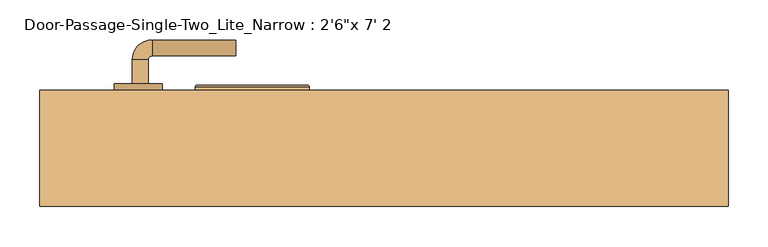
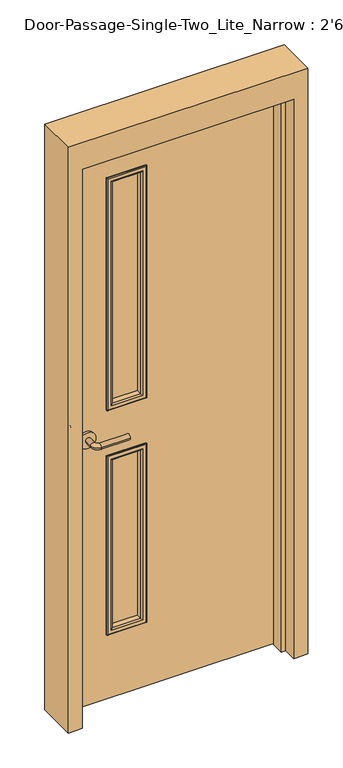
"""IFC4 building model written with IfcOpenShell, lengths in millimetres: door geometry."""

from ifc_helpers import new_model, si_unit, point, frame, frame_2d, origin, place, context, project, spatial, polyline, circle_curve, ellipse_curve, trimmed, segment, composite_curve, outline, extrude, faceted_brep, source, transform, mapped, element, save
from ifc_brep_helpers import plane_surface, cylinder_surface, revolved_surface, advanced_brep


def door_6f870c18(model_context):
    return source(origin(), model_context, "Body", "SolidModel", [
        advanced_brep(
        [(-315.990625, 42.8, 1016.0), (-295.990625, 42.8, 1016.0), (-295.990625, 12.8, 1016.0), (-315.990625, 12.8, 1016.0), (-290.990625, 7.8, 1016.0), (-290.990625, -12.2, 1016.0), (-185.990625, -12.2, 1016.0), (-185.990625, 7.8, 1016.0)],
        [
            (0, 1, circle_curve(frame((-305.990625, 42.8, 1016.0), z_axis=(0.0, 1.0, 0.0), x_axis=(1.0, 0.0, 0.0)), 10.0)),
            (1, 0, circle_curve(frame((-305.990625, 42.8, 1016.0), z_axis=(0.0, 1.0, 0.0), x_axis=(1.0, 0.0, 0.0)), 10.0)),
            (1, 2),
            (2, 3, circle_curve(frame((-305.990625, 12.8, 1016.0), z_axis=(0.0, 1.0, 0.0), x_axis=(1.0, 0.0, 0.0)), 10.0)),
            (3, 0),
            (3, 2, circle_curve(frame((-305.990625, 12.8, 1016.0), z_axis=(0.0, 1.0, 0.0), x_axis=(1.0, 0.0, 0.0)), 10.0)),
            (4, 5, circle_curve(frame((-290.990625, -2.2, 1016.0), z_axis=(-1.0, 0.0, 0.0), x_axis=(0.0, 1.0, 0.0)), 10.0)),
            (5, 3, circle_curve(frame((-290.990625, 12.8, 1016.0), z_axis=(0.0, 0.0, -1.0), x_axis=(-1.0, 0.0, 0.0)), 25.0)),
            (2, 4, circle_curve(frame((-290.990625, 12.8, 1016.0), z_axis=(0.0, 0.0, 1.0), x_axis=(-1.0, 0.0, 0.0)), 5.0)),
            (5, 4, circle_curve(frame((-290.990625, -2.2, 1016.0), z_axis=(-1.0, 0.0, 0.0), x_axis=(0.0, 1.0, 0.0)), 10.0)),
            (6, 7, circle_curve(frame((-185.990625, -2.2, 1016.0), z_axis=(1.0, 0.0, 0.0), x_axis=(0.0, 1.0, 0.0)), 10.0)),
            (7, 6, circle_curve(frame((-185.990625, -2.2, 1016.0), z_axis=(1.0, 0.0, 0.0), x_axis=(0.0, 1.0, 0.0)), 10.0)),
            (4, 7),
            (6, 5),
        ],
        [
            plane_surface(frame((-305.990625, 42.8, 1016.0), z_axis=(0.0, 1.0, 0.0), x_axis=(0.0, 0.0, 1.0))),
            cylinder_surface(frame((-305.990625, 42.8, 1016.0), z_axis=(0.0, 1.0, 0.0), x_axis=(1.0, 0.0, 0.0)), 10.0),
            revolved_surface(trimmed(ellipse_curve(frame((-305.990625, 12.8, 1016.0), z_axis=(0.0, -1.0, 0.0), x_axis=(1.0, 0.0, 0.0)), 10.0, 10.0), [point((-315.990625, 12.8, 1016.0))], [point((-295.990625, 12.8, 1016.0))], True, "CARTESIAN"), (-290.990625, 12.8, 1016.0), (0.0, 0.0, -1.0)),
            revolved_surface(trimmed(ellipse_curve(frame((-305.990625, 12.8, 1016.0), z_axis=(0.0, -1.0, 0.0), x_axis=(1.0, 0.0, 0.0)), 10.0, 10.0), [point((-295.990625, 12.8, 1016.0))], [point((-315.990625, 12.8, 1016.0))], True, "CARTESIAN"), (-290.990625, 12.8, 1016.0), (0.0, 0.0, -1.0)),
            plane_surface(frame((-185.990625, -2.2, 1016.0), z_axis=(1.0, 0.0, 0.0), x_axis=(0.0, 0.0, 1.0))),
            cylinder_surface(frame((-290.990625, -2.2, 1016.0), z_axis=(-1.0, 0.0, 0.0), x_axis=(0.0, 1.0, 0.0)), 10.0),
        ],
        [
            (0, [[1, 2]]),
            (1, [[3, 4, 5, -2]]),
            (1, [[-5, 6, -3, -1]]),
            (2, [[7, 8, -4, 9]]),
            (3, [[10, -9, -6, -8]]),
            (4, [[11, 12]]),
            (5, [[13, -11, 14, -7]]),
            (5, [[-14, -12, -13, -10]]),
        ],
    ),
        extrude(outline(composite_curve([segment(trimmed(circle_curve(frame_2d((1016.0, -308.490625)), 30.0), [point((1016.0, -338.490625))], [point((1016.0, -278.490625))], False, "CARTESIAN"), True, "CONTINUOUS"), segment(trimmed(circle_curve(frame_2d((1016.0, -308.490625)), 30.0), [point((1016.0, -278.490625))], [point((1016.0, -338.490625))], False, "CARTESIAN"), True, "CONTINUOUS")], self_intersect=False)), frame((0.0, 42.8, 0.0), z_axis=(0.0, 1.0, 0.0), x_axis=(0.0, 0.0, 1.0)), (0.0, 0.0, 1.0), 8.0),
        advanced_brep(
        [(-315.990625, 103.25, 1016.0), (-295.990625, 103.25, 1016.0), (-315.990625, 133.25, 1016.0), (-295.990625, 133.25, 1016.0), (-290.990625, 138.25, 1016.0), (-290.990625, 158.25, 1016.0), (-185.990625, 158.25, 1016.0), (-185.990625, 138.25, 1016.0)],
        [
            (0, 1, circle_curve(frame((-305.990625, 103.25, 1016.0), z_axis=(0.0, -1.0, 0.0), x_axis=(1.0, 0.0, 0.0)), 10.0)),
            (1, 0, circle_curve(frame((-305.990625, 103.25, 1016.0), z_axis=(0.0, -1.0, 0.0), x_axis=(1.0, 0.0, 0.0)), 10.0)),
            (0, 2),
            (2, 3, circle_curve(frame((-305.990625, 133.25, 1016.0), z_axis=(0.0, -1.0, 0.0), x_axis=(1.0, 0.0, 0.0)), 10.0)),
            (3, 1),
            (3, 2, circle_curve(frame((-305.990625, 133.25, 1016.0), z_axis=(0.0, -1.0, 0.0), x_axis=(1.0, 0.0, 0.0)), 10.0)),
            (4, 3, circle_curve(frame((-290.990625, 133.25, 1016.0), z_axis=(0.0, 0.0, 1.0), x_axis=(-1.0, 0.0, 0.0)), 5.0)),
            (2, 5, circle_curve(frame((-290.990625, 133.25, 1016.0), z_axis=(0.0, 0.0, -1.0), x_axis=(-1.0, 0.0, 0.0)), 25.0)),
            (5, 4, circle_curve(frame((-290.990625, 148.25, 1016.0), z_axis=(-1.0, 0.0, 0.0), x_axis=(0.0, -1.0, 0.0)), 10.0)),
            (4, 5, circle_curve(frame((-290.990625, 148.25, 1016.0), z_axis=(-1.0, 0.0, 0.0), x_axis=(0.0, -1.0, 0.0)), 10.0)),
            (6, 7, circle_curve(frame((-185.990625, 148.25, 1016.0), z_axis=(1.0, 0.0, 0.0), x_axis=(0.0, -1.0, 0.0)), 10.0)),
            (7, 6, circle_curve(frame((-185.990625, 148.25, 1016.0), z_axis=(1.0, 0.0, 0.0), x_axis=(0.0, -1.0, 0.0)), 10.0)),
            (5, 6),
            (7, 4),
        ],
        [
            plane_surface(frame((-305.990625, 103.25, 1016.0), z_axis=(0.0, -1.0, 0.0), x_axis=(0.0, 0.0, 1.0))),
            cylinder_surface(frame((-305.990625, 103.25, 1016.0), z_axis=(0.0, -1.0, 0.0), x_axis=(1.0, 0.0, 0.0)), 10.0),
            revolved_surface(trimmed(ellipse_curve(frame((-305.990625, 133.25, 1016.0), z_axis=(0.0, -1.0, 0.0), x_axis=(1.0, 0.0, 0.0)), 10.0, 10.0), [point((-315.990625, 133.25, 1016.0))], [point((-295.990625, 133.25, 1016.0))], True, "CARTESIAN"), (-290.990625, 133.25, 1016.0), (0.0, 0.0, -1.0)),
            revolved_surface(trimmed(ellipse_curve(frame((-305.990625, 133.25, 1016.0), z_axis=(0.0, -1.0, 0.0), x_axis=(1.0, 0.0, 0.0)), 10.0, 10.0), [point((-295.990625, 133.25, 1016.0))], [point((-315.990625, 133.25, 1016.0))], True, "CARTESIAN"), (-290.990625, 133.25, 1016.0), (0.0, 0.0, -1.0)),
            plane_surface(frame((-185.990625, 148.25, 1016.0), z_axis=(1.0, 0.0, 0.0), x_axis=(0.0, 0.0, 1.0))),
            cylinder_surface(frame((-290.990625, 148.25, 1016.0), z_axis=(-1.0, 0.0, 0.0), x_axis=(0.0, -1.0, 0.0)), 10.0),
        ],
        [
            (0, [[1, 2]]),
            (1, [[-1, 3, 4, 5]]),
            (1, [[-2, -5, 6, -3]]),
            (2, [[7, -4, 8, 9]]),
            (3, [[-8, -6, -7, 10]]),
            (4, [[11, 12]]),
            (5, [[-9, 13, -12, 14]]),
            (5, [[-10, -14, -11, -13]]),
        ],
    ),
        extrude(outline(composite_curve([segment(trimmed(circle_curve(frame_2d((1016.0, -308.490625)), 30.0), [point((1016.0, -338.490625))], [point((1016.0, -278.490625))], False, "CARTESIAN"), True, "CONTINUOUS"), segment(trimmed(circle_curve(frame_2d((1016.0, -308.490625)), 30.0), [point((1016.0, -278.490625))], [point((1016.0, -338.490625))], False, "CARTESIAN"), True, "CONTINUOUS")], self_intersect=False)), frame((0.0, 95.25, 0.0), z_axis=(0.0, 1.0, 0.0), x_axis=(0.0, 0.0, 1.0)), (0.0, 0.0, 1.0), 8.0),
        extrude(outline(polyline([(2133.6, -381.0), (0.0, -381.0), (0.0, 381.0), (2133.6, 381.0), (2133.6, -381.0)]), holes=[polyline([(1981.2, -228.6), (1981.2, -101.6), (1111.25, -101.6), (1111.25, -228.6), (1981.2, -228.6)]), polyline([(920.75, -228.6), (920.75, -101.6), (254.0, -101.6), (254.0, -228.6), (920.75, -228.6)])]), frame((0.0, 50.8, 0.0), z_axis=(0.0, 1.0, 0.0), x_axis=(0.0, 0.0, 1.0)), (0.0, 0.0, 1.0), 44.45),
        faceted_brep([(381.0, 46.0375, 0.0), (381.0, 95.25, 0.0), (431.8, 95.25, 0.0), (431.8, -50.8, 0.0), (381.0, -50.8, 0.0), (381.0, -1.5875, 0.0), (365.125, -1.5875, 0.0), (365.125, 46.0375, 0.0), (381.0, 46.0375, 2133.6), (381.0, 95.25, 2133.6), (-381.0, 95.25, 2133.6), (-381.0, 95.25, 0.0), (-431.8, 95.25, 0.0), (-431.8, 95.25, 2235.2), (431.8, 95.25, 2235.2), (431.8, -50.8, 2235.2), (-431.8, -50.8, 2235.2), (-431.8, -50.8, 0.0), (-381.0, -50.8, 0.0), (-381.0, -50.8, 2133.6), (381.0, -50.8, 2133.6), (381.0, -1.5875, 2133.6), (-381.0, -1.5875, 2133.6), (-381.0, -1.5875, 0.0), (-365.125, -1.5875, 0.0), (-365.125, -1.5875, 2117.725), (365.125, -1.5875, 2117.725), (365.125, 46.0375, 2117.725), (-365.125, 46.0375, 2117.725), (-365.125, 46.0375, 0.0), (-381.0, 46.0375, 0.0), (-381.0, 46.0375, 2133.6)], [[[0, 1, 2, 3, 4, 5, 6, 7]], [[1, 0, 8, 9]], [[2, 1, 9, 10, 11, 12, 13, 14]], [[3, 2, 14, 15]], [[4, 3, 15, 16, 17, 18, 19, 20]], [[5, 4, 20, 21]], [[6, 5, 21, 22, 23, 24, 25, 26]], [[7, 6, 26, 27]], [[0, 7, 27, 28, 29, 30, 31, 8]], [[9, 8, 31, 10]], [[20, 19, 22, 21]], [[26, 25, 28, 27]], [[12, 11, 30, 29, 24, 23, 18, 17]], [[11, 10, 31, 30]], [[13, 12, 17, 16]], [[19, 18, 23, 22]], [[25, 24, 29, 28]], [[15, 14, 13, 16]]]),
        extrude(outline(polyline([(-101.6, 69.85), (-228.6, 69.85), (-228.6, 76.2), (-101.6, 76.2), (-101.6, 69.85)])), frame((0.0, 0.0, 1111.25), z_axis=(0.0, 0.0, 1.0), x_axis=(1.0, 0.0, 0.0)), (0.0, 0.0, 1.0), 869.95),
        extrude(outline(polyline([(-101.6, 69.85), (-228.6, 69.85), (-228.6, 76.2), (-101.6, 76.2), (-101.6, 69.85)])), frame((0.0, 0.0, 254.0), z_axis=(0.0, 0.0, 1.0), x_axis=(1.0, 0.0, 0.0)), (0.0, 0.0, 1.0), 666.75),
        advanced_brep(
        [(-228.6, 76.2, 1981.2), (-228.6, 95.25, 1981.2), (-228.6, 95.25, 1111.25), (-228.6, 76.2, 1111.25), (-216.6, 96.25, 1969.2), (-216.6, 76.2, 1969.2), (-216.6, 76.2, 1123.25), (-216.6, 96.25, 1123.25), (-221.6, 101.25, 1974.2), (-221.6, 101.25, 1118.25), (-236.6, 99.25, 1989.2), (-234.6, 101.25, 1987.2), (-234.6, 101.25, 1105.25), (-236.6, 99.25, 1103.25), (-236.6, 95.25, 1989.2), (-236.6, 95.25, 1103.25), (-101.6, 95.25, 1111.25), (-101.6, 76.2, 1111.25), (-113.6, 76.2, 1123.25), (-113.6, 96.25, 1123.25), (-108.6, 101.25, 1118.25), (-95.6, 101.25, 1105.25), (-93.6, 99.25, 1103.25), (-93.6, 95.25, 1103.25), (-101.6, 95.25, 1981.2), (-101.6, 76.2, 1981.2), (-113.6, 76.2, 1969.2), (-113.6, 96.25, 1969.2), (-108.6, 101.25, 1974.2), (-95.6, 101.25, 1987.2), (-93.6, 99.25, 1989.2), (-93.6, 95.25, 1989.2)],
        [
            (0, 1),
            (1, 2),
            (2, 3),
            (3, 0),
            (4, 5),
            (5, 6),
            (6, 7),
            (7, 4),
            (8, 4, ellipse_curve(frame((-221.6, 96.25, 1974.2), z_axis=(-0.7071067811865475, 0.0, -0.7071067811865475), x_axis=(-0.7071067811865474, 0.0, 0.7071067811865476)), 7.0710678, 5.0)),
            (7, 9, ellipse_curve(frame((-221.6, 96.25, 1118.25), z_axis=(-0.7071067811865475, 0.0, 0.7071067811865475), x_axis=(0.7071067811865474, 0.0, 0.7071067811865476)), 7.0710678, 5.0)),
            (9, 8),
            (10, 11, ellipse_curve(frame((-234.6, 99.25, 1987.2), z_axis=(-0.7071067811865475, 0.0, -0.7071067811865475), x_axis=(-0.7071067811865474, 0.0, 0.7071067811865476)), 2.8284271, 2.0)),
            (11, 12),
            (12, 13, ellipse_curve(frame((-234.6, 99.25, 1105.25), z_axis=(-0.7071067811865475, 0.0, 0.7071067811865475), x_axis=(0.7071067811865474, 0.0, 0.7071067811865476)), 2.8284271, 2.0)),
            (13, 10),
            (14, 10),
            (13, 15),
            (15, 14),
            (2, 16),
            (16, 17),
            (17, 3),
            (6, 18),
            (18, 19),
            (19, 7),
            (19, 20, ellipse_curve(frame((-108.6, 96.25, 1118.25), z_axis=(-0.7071067811865475, 0.0, -0.7071067811865475), x_axis=(-0.7071067811865476, 0.0, 0.7071067811865474)), 7.0710678, 5.0)),
            (20, 9),
            (12, 21),
            (21, 22, ellipse_curve(frame((-95.6, 99.25, 1105.25), z_axis=(-0.7071067811865475, 0.0, -0.7071067811865475), x_axis=(-0.7071067811865476, 0.0, 0.7071067811865474)), 2.8284271, 2.0)),
            (22, 13),
            (22, 23),
            (23, 15),
            (16, 24),
            (24, 25),
            (25, 17),
            (18, 26),
            (26, 27),
            (27, 19),
            (27, 28, ellipse_curve(frame((-108.6, 96.25, 1974.2), z_axis=(0.7071067811865475, 0.0, -0.7071067811865475), x_axis=(-0.7071067811865474, 0.0, -0.7071067811865476)), 7.0710678, 5.0)),
            (28, 20),
            (21, 29),
            (29, 30, ellipse_curve(frame((-95.6, 99.25, 1987.2), z_axis=(0.7071067811865475, 0.0, -0.7071067811865475), x_axis=(-0.7071067811865474, 0.0, -0.7071067811865476)), 2.8284271, 2.0)),
            (30, 22),
            (30, 31),
            (31, 23),
            (31, 14),
            (1, 24),
            (0, 25),
            (5, 26),
            (4, 27),
            (8, 28),
            (11, 29),
            (10, 30),
        ],
        [
            plane_surface(frame((-228.6, 95.25, 1981.2), z_axis=(-1.0, 0.0, 0.0), x_axis=(0.0, 0.0, -1.0))),
            plane_surface(frame((-216.6, 76.2, 1969.2), z_axis=(1.0, 0.0, 0.0), x_axis=(0.0, 0.0, -1.0))),
            cylinder_surface(frame((-221.6, 96.25, 1981.2), z_axis=(0.0, 0.0, 1.0), x_axis=(-1.0, 0.0, 0.0)), 5.0),
            cylinder_surface(frame((-234.6, 99.25, 1981.2), z_axis=(0.0, 0.0, 1.0), x_axis=(-1.0, 0.0, 0.0)), 2.0),
            plane_surface(frame((-236.6, 99.25, 1989.2), z_axis=(-1.0, 0.0, 0.0), x_axis=(0.0, 0.0, -1.0))),
            plane_surface(frame((-228.6, 95.25, 1111.25), z_axis=(0.0, 0.0, -1.0), x_axis=(1.0, 0.0, 0.0))),
            plane_surface(frame((-216.6, 76.2, 1123.25), z_axis=(0.0, 0.0, 1.0), x_axis=(1.0, 0.0, 0.0))),
            cylinder_surface(frame((-228.6, 96.25, 1118.25), z_axis=(-1.0, 0.0, 0.0), x_axis=(0.0, 0.0, -1.0)), 5.0),
            cylinder_surface(frame((-228.6, 99.25, 1105.25), z_axis=(-1.0, 0.0, 0.0), x_axis=(0.0, 0.0, -1.0)), 2.0),
            plane_surface(frame((-236.6, 99.25, 1103.25), z_axis=(0.0, 0.0, -1.0), x_axis=(1.0, 0.0, 0.0))),
            plane_surface(frame((-101.6, 95.25, 1111.25), z_axis=(1.0, 0.0, 0.0), x_axis=(0.0, 0.0, 1.0))),
            plane_surface(frame((-113.6, 76.2, 1123.25), z_axis=(-1.0, 0.0, 0.0), x_axis=(0.0, 0.0, 1.0))),
            cylinder_surface(frame((-108.6, 96.25, 1111.25), z_axis=(0.0, 0.0, -1.0), x_axis=(1.0, 0.0, 0.0)), 5.0),
            cylinder_surface(frame((-95.6, 99.25, 1111.25), z_axis=(0.0, 0.0, -1.0), x_axis=(1.0, 0.0, 0.0)), 2.0),
            plane_surface(frame((-93.6, 99.25, 1103.25), z_axis=(1.0, 0.0, 0.0), x_axis=(0.0, 0.0, 1.0))),
            plane_surface(frame((-93.6, 95.25, 1989.2), z_axis=(0.0, -1.0, 0.0), x_axis=(-1.0, 0.0, 0.0))),
            plane_surface(frame((-101.6, 95.25, 1981.2), z_axis=(0.0, 0.0, 1.0), x_axis=(-1.0, 0.0, 0.0))),
            plane_surface(frame((-101.6, 76.2, 1981.2), z_axis=(0.0, -1.0, 0.0), x_axis=(-1.0, 0.0, 0.0))),
            plane_surface(frame((-113.6, 76.2, 1969.2), z_axis=(0.0, 0.0, -1.0), x_axis=(-1.0, 0.0, 0.0))),
            cylinder_surface(frame((-101.6, 96.25, 1974.2), z_axis=(1.0, 0.0, 0.0), x_axis=(0.0, 0.0, 1.0)), 5.0),
            plane_surface(frame((-108.6, 101.25, 1974.2), z_axis=(0.0, 1.0, 0.0), x_axis=(-1.0, 0.0, 0.0))),
            cylinder_surface(frame((-101.6, 99.25, 1987.2), z_axis=(1.0, 0.0, 0.0), x_axis=(0.0, 0.0, 1.0)), 2.0),
            plane_surface(frame((-93.6, 99.25, 1989.2), z_axis=(0.0, 0.0, 1.0), x_axis=(-1.0, 0.0, 0.0))),
        ],
        [
            (0, [[1, 2, 3, 4]]),
            (1, [[5, 6, 7, 8]]),
            (2, [[9, -8, 10, 11]]),
            (3, [[12, 13, 14, 15]]),
            (4, [[16, -15, 17, 18]]),
            (5, [[-3, 19, 20, 21]]),
            (6, [[-7, 22, 23, 24]]),
            (7, [[-10, -24, 25, 26]]),
            (8, [[-14, 27, 28, 29]]),
            (9, [[-17, -29, 30, 31]]),
            (10, [[-20, 32, 33, 34]]),
            (11, [[-23, 35, 36, 37]]),
            (12, [[-25, -37, 38, 39]]),
            (13, [[-28, 40, 41, 42]]),
            (14, [[-30, -42, 43, 44]]),
            (15, [[-31, -44, 45, -18], [46, -32, -19, -2]]),
            (16, [[-33, -46, -1, 47]]),
            (17, [[-21, -34, -47, -4], [48, -35, -22, -6]]),
            (18, [[-36, -48, -5, 49]]),
            (19, [[-38, -49, -9, 50]]),
            (20, [[51, -40, -27, -13], [-26, -39, -50, -11]]),
            (21, [[-41, -51, -12, 52]]),
            (22, [[-43, -52, -16, -45]]),
        ],
    ),
        advanced_brep(
        [(-228.6, 69.85, 1111.25), (-228.6, 50.8, 1111.25), (-228.6, 50.8, 1981.2), (-228.6, 69.85, 1981.2), (-216.6, 49.8, 1123.25), (-216.6, 69.85, 1123.25), (-216.6, 69.85, 1969.2), (-216.6, 49.8, 1969.2), (-221.6, 44.8, 1118.25), (-221.6, 44.8, 1974.2), (-236.6, 46.8, 1103.25), (-234.6, 44.8, 1105.25), (-234.6, 44.8, 1987.2), (-236.6, 46.8, 1989.2), (-236.6, 50.8, 1103.25), (-236.6, 50.8, 1989.2), (-101.6, 50.8, 1981.2), (-101.6, 69.85, 1981.2), (-113.6, 69.85, 1969.2), (-113.6, 49.8, 1969.2), (-108.6, 44.8, 1974.2), (-95.6, 44.8, 1987.2), (-93.6, 46.8, 1989.2), (-93.6, 50.8, 1989.2), (-101.6, 50.8, 1111.25), (-101.6, 69.85, 1111.25), (-113.6, 69.85, 1123.25), (-113.6, 49.8, 1123.25), (-108.6, 44.8, 1118.25), (-95.6, 44.8, 1105.25), (-93.6, 46.8, 1103.25), (-93.6, 50.8, 1103.25)],
        [
            (0, 1),
            (1, 2),
            (2, 3),
            (3, 0),
            (4, 5),
            (5, 6),
            (6, 7),
            (7, 4),
            (8, 4, ellipse_curve(frame((-221.6, 49.8, 1118.25), z_axis=(-0.7071067811865475, 0.0, 0.7071067811865475), x_axis=(-0.7071067811865474, 0.0, -0.7071067811865476)), 7.0710678, 5.0)),
            (7, 9, ellipse_curve(frame((-221.6, 49.8, 1974.2), z_axis=(-0.7071067811865475, 0.0, -0.7071067811865475), x_axis=(0.7071067811865474, 0.0, -0.7071067811865476)), 7.0710678, 5.0)),
            (9, 8),
            (10, 11, ellipse_curve(frame((-234.6, 46.8, 1105.25), z_axis=(-0.7071067811865475, 0.0, 0.7071067811865475), x_axis=(-0.7071067811865474, 0.0, -0.7071067811865476)), 2.8284271, 2.0)),
            (11, 12),
            (12, 13, ellipse_curve(frame((-234.6, 46.8, 1987.2), z_axis=(-0.7071067811865475, 0.0, -0.7071067811865475), x_axis=(0.7071067811865474, 0.0, -0.7071067811865476)), 2.8284271, 2.0)),
            (13, 10),
            (14, 10),
            (13, 15),
            (15, 14),
            (2, 16),
            (16, 17),
            (17, 3),
            (6, 18),
            (18, 19),
            (19, 7),
            (19, 20, ellipse_curve(frame((-108.6, 49.8, 1974.2), z_axis=(-0.7071067811865475, 0.0, 0.7071067811865475), x_axis=(-0.7071067811865476, 0.0, -0.7071067811865474)), 7.0710678, 5.0)),
            (20, 9),
            (12, 21),
            (21, 22, ellipse_curve(frame((-95.6, 46.8, 1987.2), z_axis=(-0.7071067811865475, 0.0, 0.7071067811865475), x_axis=(-0.7071067811865476, 0.0, -0.7071067811865474)), 2.8284271, 2.0)),
            (22, 13),
            (22, 23),
            (23, 15),
            (16, 24),
            (24, 25),
            (25, 17),
            (18, 26),
            (26, 27),
            (27, 19),
            (27, 28, ellipse_curve(frame((-108.6, 49.8, 1118.25), z_axis=(0.7071067811865475, 0.0, 0.7071067811865475), x_axis=(-0.7071067811865474, 0.0, 0.7071067811865476)), 7.0710678, 5.0)),
            (28, 20),
            (21, 29),
            (29, 30, ellipse_curve(frame((-95.6, 46.8, 1105.25), z_axis=(0.7071067811865475, 0.0, 0.7071067811865475), x_axis=(-0.7071067811865474, 0.0, 0.7071067811865476)), 2.8284271, 2.0)),
            (30, 22),
            (30, 31),
            (31, 23),
            (31, 14),
            (1, 24),
            (0, 25),
            (5, 26),
            (4, 27),
            (8, 28),
            (11, 29),
            (10, 30),
        ],
        [
            plane_surface(frame((-228.6, 50.8, 1111.25), z_axis=(-1.0, 0.0, 0.0), x_axis=(0.0, 0.0, 1.0))),
            plane_surface(frame((-216.6, 69.85, 1123.25), z_axis=(1.0, 0.0, 0.0), x_axis=(0.0, 0.0, 1.0))),
            cylinder_surface(frame((-221.6, 49.8, 1111.25), z_axis=(0.0, 0.0, -1.0), x_axis=(-1.0, 0.0, 0.0)), 5.0),
            cylinder_surface(frame((-234.6, 46.8, 1111.25), z_axis=(0.0, 0.0, -1.0), x_axis=(-1.0, 0.0, 0.0)), 2.0),
            plane_surface(frame((-236.6, 46.8, 1103.25), z_axis=(-1.0, 0.0, 0.0), x_axis=(0.0, 0.0, 1.0))),
            plane_surface(frame((-228.6, 50.8, 1981.2), z_axis=(0.0, 0.0, 1.0), x_axis=(1.0, 0.0, 0.0))),
            plane_surface(frame((-216.6, 69.85, 1969.2), z_axis=(0.0, 0.0, -1.0), x_axis=(1.0, 0.0, 0.0))),
            cylinder_surface(frame((-228.6, 49.8, 1974.2), z_axis=(-1.0, 0.0, 0.0), x_axis=(0.0, 0.0, 1.0)), 5.0),
            cylinder_surface(frame((-228.6, 46.8, 1987.2), z_axis=(-1.0, 0.0, 0.0), x_axis=(0.0, 0.0, 1.0)), 2.0),
            plane_surface(frame((-236.6, 46.8, 1989.2), z_axis=(0.0, 0.0, 1.0), x_axis=(1.0, 0.0, 0.0))),
            plane_surface(frame((-101.6, 50.8, 1981.2), z_axis=(1.0, 0.0, 0.0), x_axis=(0.0, 0.0, -1.0))),
            plane_surface(frame((-113.6, 69.85, 1969.2), z_axis=(-1.0, 0.0, 0.0), x_axis=(0.0, 0.0, -1.0))),
            cylinder_surface(frame((-108.6, 49.8, 1981.2), z_axis=(0.0, 0.0, 1.0), x_axis=(1.0, 0.0, 0.0)), 5.0),
            cylinder_surface(frame((-95.6, 46.8, 1981.2), z_axis=(0.0, 0.0, 1.0), x_axis=(1.0, 0.0, 0.0)), 2.0),
            plane_surface(frame((-93.6, 46.8, 1989.2), z_axis=(1.0, 0.0, 0.0), x_axis=(0.0, 0.0, -1.0))),
            plane_surface(frame((-93.6, 50.8, 1103.25), z_axis=(0.0, 1.0, 0.0), x_axis=(-1.0, 0.0, 0.0))),
            plane_surface(frame((-101.6, 50.8, 1111.25), z_axis=(0.0, 0.0, -1.0), x_axis=(-1.0, 0.0, 0.0))),
            plane_surface(frame((-101.6, 69.85, 1111.25), z_axis=(0.0, 1.0, 0.0), x_axis=(-1.0, 0.0, 0.0))),
            plane_surface(frame((-113.6, 69.85, 1123.25), z_axis=(0.0, 0.0, 1.0), x_axis=(-1.0, 0.0, 0.0))),
            cylinder_surface(frame((-101.6, 49.8, 1118.25), z_axis=(1.0, 0.0, 0.0), x_axis=(0.0, 0.0, -1.0)), 5.0),
            plane_surface(frame((-108.6, 44.8, 1118.25), z_axis=(0.0, -1.0, 0.0), x_axis=(-1.0, 0.0, 0.0))),
            cylinder_surface(frame((-101.6, 46.8, 1105.25), z_axis=(1.0, 0.0, 0.0), x_axis=(0.0, 0.0, -1.0)), 2.0),
            plane_surface(frame((-93.6, 46.8, 1103.25), z_axis=(0.0, 0.0, -1.0), x_axis=(-1.0, 0.0, 0.0))),
        ],
        [
            (0, [[1, 2, 3, 4]]),
            (1, [[5, 6, 7, 8]]),
            (2, [[9, -8, 10, 11]]),
            (3, [[12, 13, 14, 15]]),
            (4, [[16, -15, 17, 18]]),
            (5, [[-3, 19, 20, 21]]),
            (6, [[-7, 22, 23, 24]]),
            (7, [[-10, -24, 25, 26]]),
            (8, [[-14, 27, 28, 29]]),
            (9, [[-17, -29, 30, 31]]),
            (10, [[-20, 32, 33, 34]]),
            (11, [[-23, 35, 36, 37]]),
            (12, [[-25, -37, 38, 39]]),
            (13, [[-28, 40, 41, 42]]),
            (14, [[-30, -42, 43, 44]]),
            (15, [[-31, -44, 45, -18], [46, -32, -19, -2]]),
            (16, [[-33, -46, -1, 47]]),
            (17, [[-21, -34, -47, -4], [48, -35, -22, -6]]),
            (18, [[-36, -48, -5, 49]]),
            (19, [[-38, -49, -9, 50]]),
            (20, [[51, -40, -27, -13], [-26, -39, -50, -11]]),
            (21, [[-41, -51, -12, 52]]),
            (22, [[-43, -52, -16, -45]]),
        ],
    ),
        advanced_brep(
        [(-228.6, 76.2, 920.75), (-228.6, 95.25, 920.75), (-228.6, 95.25, 254.0), (-228.6, 76.2, 254.0), (-216.6, 96.25, 908.75), (-216.6, 76.2, 908.75), (-216.6, 76.2, 266.0), (-216.6, 96.25, 266.0), (-221.6, 101.25, 913.75), (-221.6, 101.25, 261.0), (-236.6, 99.25, 928.75), (-234.6, 101.25, 926.75), (-234.6, 101.25, 248.0), (-236.6, 99.25, 246.0), (-236.6, 95.25, 928.75), (-236.6, 95.25, 246.0), (-101.6, 95.25, 254.0), (-101.6, 76.2, 254.0), (-113.6, 76.2, 266.0), (-113.6, 96.25, 266.0), (-108.6, 101.25, 261.0), (-95.6, 101.25, 248.0), (-93.6, 99.25, 246.0), (-93.6, 95.25, 246.0), (-101.6, 95.25, 920.75), (-101.6, 76.2, 920.75), (-113.6, 76.2, 908.75), (-113.6, 96.25, 908.75), (-108.6, 101.25, 913.75), (-95.6, 101.25, 926.75), (-93.6, 99.25, 928.75), (-93.6, 95.25, 928.75)],
        [
            (0, 1),
            (1, 2),
            (2, 3),
            (3, 0),
            (4, 5),
            (5, 6),
            (6, 7),
            (7, 4),
            (8, 4, ellipse_curve(frame((-221.6, 96.25, 913.75), z_axis=(-0.7071067811865475, 0.0, -0.7071067811865475), x_axis=(-0.7071067811865474, 0.0, 0.7071067811865476)), 7.0710678, 5.0)),
            (7, 9, ellipse_curve(frame((-221.6, 96.25, 261.0), z_axis=(-0.7071067811865475, 0.0, 0.7071067811865475), x_axis=(0.7071067811865474, 0.0, 0.7071067811865476)), 7.0710678, 5.0)),
            (9, 8),
            (10, 11, ellipse_curve(frame((-234.6, 99.25, 926.75), z_axis=(-0.7071067811865475, 0.0, -0.7071067811865475), x_axis=(-0.7071067811865474, 0.0, 0.7071067811865476)), 2.8284271, 2.0)),
            (11, 12),
            (12, 13, ellipse_curve(frame((-234.6, 99.25, 248.0), z_axis=(-0.7071067811865475, 0.0, 0.7071067811865475), x_axis=(0.7071067811865474, 0.0, 0.7071067811865476)), 2.8284271, 2.0)),
            (13, 10),
            (14, 10),
            (13, 15),
            (15, 14),
            (2, 16),
            (16, 17),
            (17, 3),
            (6, 18),
            (18, 19),
            (19, 7),
            (19, 20, ellipse_curve(frame((-108.6, 96.25, 261.0), z_axis=(-0.7071067811865475, 0.0, -0.7071067811865475), x_axis=(-0.7071067811865476, 0.0, 0.7071067811865474)), 7.0710678, 5.0)),
            (20, 9),
            (12, 21),
            (21, 22, ellipse_curve(frame((-95.6, 99.25, 248.0), z_axis=(-0.7071067811865475, 0.0, -0.7071067811865475), x_axis=(-0.7071067811865476, 0.0, 0.7071067811865474)), 2.8284271, 2.0)),
            (22, 13),
            (22, 23),
            (23, 15),
            (16, 24),
            (24, 25),
            (25, 17),
            (18, 26),
            (26, 27),
            (27, 19),
            (27, 28, ellipse_curve(frame((-108.6, 96.25, 913.75), z_axis=(0.7071067811865475, 0.0, -0.7071067811865475), x_axis=(-0.7071067811865474, 0.0, -0.7071067811865476)), 7.0710678, 5.0)),
            (28, 20),
            (21, 29),
            (29, 30, ellipse_curve(frame((-95.6, 99.25, 926.75), z_axis=(0.7071067811865475, 0.0, -0.7071067811865475), x_axis=(-0.7071067811865474, 0.0, -0.7071067811865476)), 2.8284271, 2.0)),
            (30, 22),
            (30, 31),
            (31, 23),
            (31, 14),
            (1, 24),
            (0, 25),
            (5, 26),
            (4, 27),
            (8, 28),
            (11, 29),
            (10, 30),
        ],
        [
            plane_surface(frame((-228.6, 95.25, 920.75), z_axis=(-1.0, 0.0, 0.0), x_axis=(0.0, 0.0, -1.0))),
            plane_surface(frame((-216.6, 76.2, 908.75), z_axis=(1.0, 0.0, 0.0), x_axis=(0.0, 0.0, -1.0))),
            cylinder_surface(frame((-221.6, 96.25, 920.75), z_axis=(0.0, 0.0, 1.0), x_axis=(-1.0, 0.0, 0.0)), 5.0),
            cylinder_surface(frame((-234.6, 99.25, 920.75), z_axis=(0.0, 0.0, 1.0), x_axis=(-1.0, 0.0, 0.0)), 2.0),
            plane_surface(frame((-236.6, 99.25, 928.75), z_axis=(-1.0, 0.0, 0.0), x_axis=(0.0, 0.0, -1.0))),
            plane_surface(frame((-228.6, 95.25, 254.0), z_axis=(0.0, 0.0, -1.0), x_axis=(1.0, 0.0, 0.0))),
            plane_surface(frame((-216.6, 76.2, 266.0), z_axis=(0.0, 0.0, 1.0), x_axis=(1.0, 0.0, 0.0))),
            cylinder_surface(frame((-228.6, 96.25, 261.0), z_axis=(-1.0, 0.0, 0.0), x_axis=(0.0, 0.0, -1.0)), 5.0),
            cylinder_surface(frame((-228.6, 99.25, 248.0), z_axis=(-1.0, 0.0, 0.0), x_axis=(0.0, 0.0, -1.0)), 2.0),
            plane_surface(frame((-236.6, 99.25, 246.0), z_axis=(0.0, 0.0, -1.0), x_axis=(1.0, 0.0, 0.0))),
            plane_surface(frame((-101.6, 95.25, 254.0), z_axis=(1.0, 0.0, 0.0), x_axis=(0.0, 0.0, 1.0))),
            plane_surface(frame((-113.6, 76.2, 266.0), z_axis=(-1.0, 0.0, 0.0), x_axis=(0.0, 0.0, 1.0))),
            cylinder_surface(frame((-108.6, 96.25, 254.0), z_axis=(0.0, 0.0, -1.0), x_axis=(1.0, 0.0, 0.0)), 5.0),
            cylinder_surface(frame((-95.6, 99.25, 254.0), z_axis=(0.0, 0.0, -1.0), x_axis=(1.0, 0.0, 0.0)), 2.0),
            plane_surface(frame((-93.6, 99.25, 246.0), z_axis=(1.0, 0.0, 0.0), x_axis=(0.0, 0.0, 1.0))),
            plane_surface(frame((-93.6, 95.25, 928.75), z_axis=(0.0, -1.0, 0.0), x_axis=(-1.0, 0.0, 0.0))),
            plane_surface(frame((-101.6, 95.25, 920.75), z_axis=(0.0, 0.0, 1.0), x_axis=(-1.0, 0.0, 0.0))),
            plane_surface(frame((-101.6, 76.2, 920.75), z_axis=(0.0, -1.0, 0.0), x_axis=(-1.0, 0.0, 0.0))),
            plane_surface(frame((-113.6, 76.2, 908.75), z_axis=(0.0, 0.0, -1.0), x_axis=(-1.0, 0.0, 0.0))),
            cylinder_surface(frame((-101.6, 96.25, 913.75), z_axis=(1.0, 0.0, 0.0), x_axis=(0.0, 0.0, 1.0)), 5.0),
            plane_surface(frame((-108.6, 101.25, 913.75), z_axis=(0.0, 1.0, 0.0), x_axis=(-1.0, 0.0, 0.0))),
            cylinder_surface(frame((-101.6, 99.25, 926.75), z_axis=(1.0, 0.0, 0.0), x_axis=(0.0, 0.0, 1.0)), 2.0),
            plane_surface(frame((-93.6, 99.25, 928.75), z_axis=(0.0, 0.0, 1.0), x_axis=(-1.0, 0.0, 0.0))),
        ],
        [
            (0, [[1, 2, 3, 4]]),
            (1, [[5, 6, 7, 8]]),
            (2, [[9, -8, 10, 11]]),
            (3, [[12, 13, 14, 15]]),
            (4, [[16, -15, 17, 18]]),
            (5, [[-3, 19, 20, 21]]),
            (6, [[-7, 22, 23, 24]]),
            (7, [[-10, -24, 25, 26]]),
            (8, [[-14, 27, 28, 29]]),
            (9, [[-17, -29, 30, 31]]),
            (10, [[-20, 32, 33, 34]]),
            (11, [[-23, 35, 36, 37]]),
            (12, [[-25, -37, 38, 39]]),
            (13, [[-28, 40, 41, 42]]),
            (14, [[-30, -42, 43, 44]]),
            (15, [[-31, -44, 45, -18], [46, -32, -19, -2]]),
            (16, [[-33, -46, -1, 47]]),
            (17, [[-21, -34, -47, -4], [48, -35, -22, -6]]),
            (18, [[-36, -48, -5, 49]]),
            (19, [[-38, -49, -9, 50]]),
            (20, [[51, -40, -27, -13], [-26, -39, -50, -11]]),
            (21, [[-41, -51, -12, 52]]),
            (22, [[-43, -52, -16, -45]]),
        ],
    ),
        advanced_brep(
        [(-101.6, 69.85, 920.75), (-101.6, 50.8, 920.75), (-101.6, 50.8, 254.0), (-101.6, 69.85, 254.0), (-113.6, 49.8, 908.75), (-113.6, 69.85, 908.75), (-113.6, 69.85, 266.0), (-113.6, 49.8, 266.0), (-108.6, 44.8, 913.75), (-108.6, 44.8, 261.0), (-93.6, 46.8, 928.75), (-95.6, 44.8, 926.75), (-95.6, 44.8, 248.0), (-93.6, 46.8, 246.0), (-93.6, 50.8, 928.75), (-93.6, 50.8, 246.0), (-228.6, 50.8, 254.0), (-228.6, 69.85, 254.0), (-216.6, 69.85, 266.0), (-216.6, 49.8, 266.0), (-221.6, 44.8, 261.0), (-234.6, 44.8, 248.0), (-236.6, 46.8, 246.0), (-236.6, 50.8, 246.0), (-228.6, 50.8, 920.75), (-228.6, 69.85, 920.75), (-216.6, 69.85, 908.75), (-216.6, 49.8, 908.75), (-221.6, 44.8, 913.75), (-234.6, 44.8, 926.75), (-236.6, 46.8, 928.75), (-236.6, 50.8, 928.75)],
        [
            (0, 1),
            (1, 2),
            (2, 3),
            (3, 0),
            (4, 5),
            (5, 6),
            (6, 7),
            (7, 4),
            (8, 4, ellipse_curve(frame((-108.6, 49.8, 913.75), z_axis=(0.7071067811865475, 0.0, -0.7071067811865475), x_axis=(0.7071067811865474, 0.0, 0.7071067811865476)), 7.0710678, 5.0)),
            (7, 9, ellipse_curve(frame((-108.6, 49.8, 261.0), z_axis=(0.7071067811865475, 0.0, 0.7071067811865475), x_axis=(-0.7071067811865474, 0.0, 0.7071067811865476)), 7.0710678, 5.0)),
            (9, 8),
            (10, 11, ellipse_curve(frame((-95.6, 46.8, 926.75), z_axis=(0.7071067811865475, 0.0, -0.7071067811865475), x_axis=(0.7071067811865474, 0.0, 0.7071067811865476)), 2.8284271, 2.0)),
            (11, 12),
            (12, 13, ellipse_curve(frame((-95.6, 46.8, 248.0), z_axis=(0.7071067811865475, 0.0, 0.7071067811865475), x_axis=(-0.7071067811865474, 0.0, 0.7071067811865476)), 2.8284271, 2.0)),
            (13, 10),
            (14, 10),
            (13, 15),
            (15, 14),
            (2, 16),
            (16, 17),
            (17, 3),
            (6, 18),
            (18, 19),
            (19, 7),
            (19, 20, ellipse_curve(frame((-221.6, 49.8, 261.0), z_axis=(0.7071067811865475, 0.0, -0.7071067811865475), x_axis=(0.7071067811865476, 0.0, 0.7071067811865474)), 7.0710678, 5.0)),
            (20, 9),
            (12, 21),
            (21, 22, ellipse_curve(frame((-234.6, 46.8, 248.0), z_axis=(0.7071067811865475, 0.0, -0.7071067811865475), x_axis=(0.7071067811865476, 0.0, 0.7071067811865474)), 2.8284271, 2.0)),
            (22, 13),
            (22, 23),
            (23, 15),
            (16, 24),
            (24, 25),
            (25, 17),
            (18, 26),
            (26, 27),
            (27, 19),
            (27, 28, ellipse_curve(frame((-221.6, 49.8, 913.75), z_axis=(-0.7071067811865475, 0.0, -0.7071067811865475), x_axis=(0.7071067811865474, 0.0, -0.7071067811865476)), 7.0710678, 5.0)),
            (28, 20),
            (21, 29),
            (29, 30, ellipse_curve(frame((-234.6, 46.8, 926.75), z_axis=(-0.7071067811865475, 0.0, -0.7071067811865475), x_axis=(0.7071067811865474, 0.0, -0.7071067811865476)), 2.8284271, 2.0)),
            (30, 22),
            (30, 31),
            (31, 23),
            (31, 14),
            (1, 24),
            (0, 25),
            (5, 26),
            (4, 27),
            (8, 28),
            (11, 29),
            (10, 30),
        ],
        [
            plane_surface(frame((-101.6, 50.8, 920.75), z_axis=(1.0, 0.0, 0.0), x_axis=(0.0, 0.0, -1.0))),
            plane_surface(frame((-113.6, 69.85, 908.75), z_axis=(-1.0, 0.0, 0.0), x_axis=(0.0, 0.0, -1.0))),
            cylinder_surface(frame((-108.6, 49.8, 920.75), z_axis=(0.0, 0.0, 1.0), x_axis=(1.0, 0.0, 0.0)), 5.0),
            cylinder_surface(frame((-95.6, 46.8, 920.75), z_axis=(0.0, 0.0, 1.0), x_axis=(1.0, 0.0, 0.0)), 2.0),
            plane_surface(frame((-93.6, 46.8, 928.75), z_axis=(1.0, 0.0, 0.0), x_axis=(0.0, 0.0, -1.0))),
            plane_surface(frame((-101.6, 50.8, 254.0), z_axis=(0.0, 0.0, -1.0), x_axis=(-1.0, 0.0, 0.0))),
            plane_surface(frame((-113.6, 69.85, 266.0), z_axis=(0.0, 0.0, 1.0), x_axis=(-1.0, 0.0, 0.0))),
            cylinder_surface(frame((-101.6, 49.8, 261.0), z_axis=(1.0, 0.0, 0.0), x_axis=(0.0, 0.0, -1.0)), 5.0),
            cylinder_surface(frame((-101.6, 46.8, 248.0), z_axis=(1.0, 0.0, 0.0), x_axis=(0.0, 0.0, -1.0)), 2.0),
            plane_surface(frame((-93.6, 46.8, 246.0), z_axis=(0.0, 0.0, -1.0), x_axis=(-1.0, 0.0, 0.0))),
            plane_surface(frame((-228.6, 50.8, 254.0), z_axis=(-1.0, 0.0, 0.0), x_axis=(0.0, 0.0, 1.0))),
            plane_surface(frame((-216.6, 69.85, 266.0), z_axis=(1.0, 0.0, 0.0), x_axis=(0.0, 0.0, 1.0))),
            cylinder_surface(frame((-221.6, 49.8, 254.0), z_axis=(0.0, 0.0, -1.0), x_axis=(-1.0, 0.0, 0.0)), 5.0),
            cylinder_surface(frame((-234.6, 46.8, 254.0), z_axis=(0.0, 0.0, -1.0), x_axis=(-1.0, 0.0, 0.0)), 2.0),
            plane_surface(frame((-236.6, 46.8, 246.0), z_axis=(-1.0, 0.0, 0.0), x_axis=(0.0, 0.0, 1.0))),
            plane_surface(frame((-236.6, 50.8, 928.75), z_axis=(0.0, 1.0, 0.0), x_axis=(1.0, 0.0, 0.0))),
            plane_surface(frame((-228.6, 50.8, 920.75), z_axis=(0.0, 0.0, 1.0), x_axis=(1.0, 0.0, 0.0))),
            plane_surface(frame((-228.6, 69.85, 920.75), z_axis=(0.0, 1.0, 0.0), x_axis=(1.0, 0.0, 0.0))),
            plane_surface(frame((-216.6, 69.85, 908.75), z_axis=(0.0, 0.0, -1.0), x_axis=(1.0, 0.0, 0.0))),
            cylinder_surface(frame((-228.6, 49.8, 913.75), z_axis=(-1.0, 0.0, 0.0), x_axis=(0.0, 0.0, 1.0)), 5.0),
            plane_surface(frame((-221.6, 44.8, 913.75), z_axis=(0.0, -1.0, 0.0), x_axis=(1.0, 0.0, 0.0))),
            cylinder_surface(frame((-228.6, 46.8, 926.75), z_axis=(-1.0, 0.0, 0.0), x_axis=(0.0, 0.0, 1.0)), 2.0),
            plane_surface(frame((-236.6, 46.8, 928.75), z_axis=(0.0, 0.0, 1.0), x_axis=(1.0, 0.0, 0.0))),
        ],
        [
            (0, [[1, 2, 3, 4]]),
            (1, [[5, 6, 7, 8]]),
            (2, [[9, -8, 10, 11]]),
            (3, [[12, 13, 14, 15]]),
            (4, [[16, -15, 17, 18]]),
            (5, [[-3, 19, 20, 21]]),
            (6, [[-7, 22, 23, 24]]),
            (7, [[-10, -24, 25, 26]]),
            (8, [[-14, 27, 28, 29]]),
            (9, [[-17, -29, 30, 31]]),
            (10, [[-20, 32, 33, 34]]),
            (11, [[-23, 35, 36, 37]]),
            (12, [[-25, -37, 38, 39]]),
            (13, [[-28, 40, 41, 42]]),
            (14, [[-30, -42, 43, 44]]),
            (15, [[-31, -44, 45, -18], [46, -32, -19, -2]]),
            (16, [[-33, -46, -1, 47]]),
            (17, [[-21, -34, -47, -4], [48, -35, -22, -6]]),
            (18, [[-36, -48, -5, 49]]),
            (19, [[-38, -49, -9, 50]]),
            (20, [[51, -40, -27, -13], [-26, -39, -50, -11]]),
            (21, [[-41, -51, -12, 52]]),
            (22, [[-43, -52, -16, -45]]),
        ],
    ),
    ])


if __name__ == "__main__":
    model = new_model("IFC4")
    model_context = context("Model", 3, world=origin())
    ifc_project = project(units=[si_unit("LENGTHUNIT", "METRE", prefix="MILLI")], contexts=[model_context])
    site = spatial("IfcSite", under=ifc_project)
    building = spatial("IfcBuilding", under=site)
    placement = place(None, origin())
    door_shape = door_6f870c18(model_context)
    element("IfcDoor", 1, ObjectType="Door-Passage-Single-Two_Lite_Narrow : 2'6\"x 7' 2", at=placement, inside=building, context=model_context, shape_type="MappedRepresentation", body=[
        mapped(door_shape, transform((0.0, 0.0, 0.0), x_axis=(1.0, 0.0, 0.0), y_axis=(0.0, 1.0, 0.0), z_axis=(0.0, 0.0, 1.0))),
    ])
    save(model, "model.ifc")

# Revit data of these elements
# Type "Door-Passage-Single-Two_Lite_Narrow : 2'6\"x 7' 2"
#   Type Mark = "10"
#   Assembly Code = "B2030100"
#   Analytic Construction = "Wooden"
#   Thickness = 0' - 1 3/4"
#   Thermal Resistance (R) = 2.5876 (h·ft²·°F)/BTU
#   Swing Angle [instance default] = 90.00°
#   Strike Height = 3' - 4"
#   Rough Width [instance default] = 2' - 10"
#   Rough Height [instance default] = 7' - 4"
#   MFOpeningHeight [instance default] = 0' - 4"
#   MFOpeningWidth [instance default] = 0' - 4"
#   Heat Transfer Coefficient (U) = 0.3865 BTU/(h·ft²·°F)
#   Inset Calculate [instance default] = 0' - 4"
#   Masonry Inset [instance default] = 0' - 1"
#   Height = 7' - 0"
#   Width = 2' - 6"
#   Masonry Frame Depth = 0' - 5 3/4"
#   Masonry Frame [instance default] = yes
#   Function = 1
#   Dry Wall Frame [instance default] = no
#   Panel Material = Wood - Birch
#   Glazing = Glass
#   Glass Stop Material = Metal - Paint Finish - Grey
#   Frame Material = Metal - Paint Finish - Grey
#   Door Handle Material = Aluminum
#   Visual Light Transmittance = 0
#   Solar Heat Gain Coefficient = 0
#   Wall Closure = (empty or 0)
# Element 1 (IfcDoor, "Door-Passage-Single-Two_Lite_Narrow : 2'6\"x 7' 2")
#   Materials on its faces: "Metal - Paint Finish - Grey", "Aluminum", "Wood - Birch", "Glass"
# Materials
#   "Wood - Birch": class "Wood", colour RGB 166 116 52, transparency 0, Cost = 0
#   "Glass": class "Glass", colour RGB 0 128 192, transparency 0.75, Description = "Soda Lime Glass", Cost = 0
#   "Metal - Paint Finish - Grey": class "Paint", colour RGB 104 104 104, transparency 0, Cost = 0
#   "Aluminum": class "Metal", colour RGB 247 247 247, transparency 0, Description = "Aluminum 6061", Cost = 0
